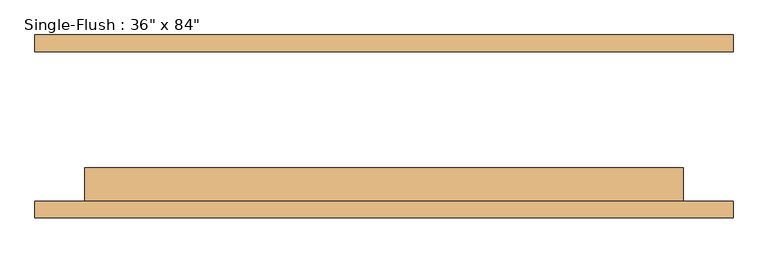
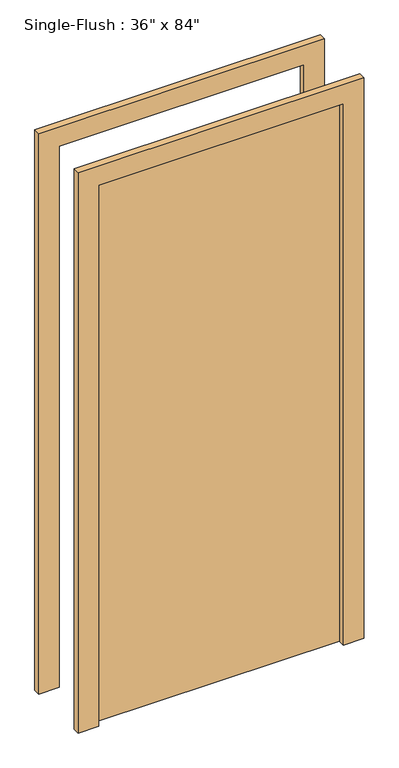
"""IFC4 building model written with IfcOpenShell, lengths in millimetres: door geometry."""

from ifc_helpers import new_model, si_unit, frame, origin, origin_with_axes, place, context, project, spatial, polyline, outline, extrude, source, transform, mapped, element, save


def door_a90ba1ad(model_context):
    return source(origin(), model_context, "Body", "SweptSolid", [
        extrude(outline(polyline([(2209.8, -533.4), (0.0, -533.4), (0.0, -457.2), (2133.6, -457.2), (2133.6, 457.2), (0.0, 457.2), (0.0, 533.4), (2209.8, 533.4), (2209.8, -533.4)])), frame((0.0, -139.7, 0.0), z_axis=(0.0, 1.0, 0.0), x_axis=(0.0, 0.0, 1.0)), (0.0, 0.0, 1.0), 25.4),
        extrude(outline(polyline([(2209.8, 533.4), (2209.8, -533.4), (0.0, -533.4), (0.0, -457.2), (2133.6, -457.2), (2133.6, 457.2), (0.0, 457.2), (0.0, 533.4), (2209.8, 533.4)])), frame((0.0, 114.3, 0.0), z_axis=(0.0, 1.0, 0.0), x_axis=(0.0, 0.0, 1.0)), (0.0, 0.0, 1.0), 25.4),
        extrude(outline(polyline([(457.2, -63.5), (457.2, -114.3), (-457.2, -114.3), (-457.2, -63.5), (457.2, -63.5)])), origin_with_axes(), (0.0, 0.0, 1.0), 2133.6),
    ])


if __name__ == "__main__":
    model = new_model("IFC4")
    model_context = context("Model", 3, world=origin())
    ifc_project = project(units=[si_unit("LENGTHUNIT", "METRE", prefix="MILLI")], contexts=[model_context])
    site = spatial("IfcSite", under=ifc_project)
    building = spatial("IfcBuilding", under=site)
    placement = place(None, origin())
    door_shape = door_a90ba1ad(model_context)
    element("IfcDoor", 1, ObjectType="Single-Flush : 36\" x 84\"", at=placement, inside=building, context=model_context, shape_type="MappedRepresentation", body=[
        mapped(door_shape, transform((0.0, 0.0, 0.0), x_axis=(1.0, 0.0, 0.0), y_axis=(0.0, 1.0, 0.0), z_axis=(0.0, 0.0, 1.0))),
    ])
    save(model, "model.ifc")

# Revit data of these elements
# Type "Single-Flush : 36\" x 84\""
#   Type Mark = "1"
#   Construction Type Id = "MDOOR"
#   Assembly Code = "C1020"
#   Analytic Construction = "Metal"
#   Thickness = 0' - 2"
#   Heat Transfer Coefficient (U) = 0.651978 BTU/(h·ft²·°F)
#   Height = 7' - 0"
#   Trim Projection Ext = 0' - 1"
#   Trim Projection Int = 0' - 1"
#   Trim Width = 0' - 3"
#   Width = 3' - 0"
#   Define Thermal Properties by = 1
#   Define Thermal Properties by = 1
#   Door Material = Door - Panel
#   Frame Material = Door - Frame
#   Visual Light Transmittance = 0
#   Solar Heat Gain Coefficient = 0
#   Function = (empty or 0)
#   Wall Closure = (empty or 0)
# Element 1 (IfcDoor, "Single-Flush : 36\" x 84\"")
#   Materials on its faces: "Door - Frame", "Door - Panel"
# Materials
#   "Door - Panel": class "Wood", colour RGB 210 159 95, transparency 0, Cost = 0
#   "Door - Frame": colour RGB 118 70 51, transparency 0, Cost = 0
